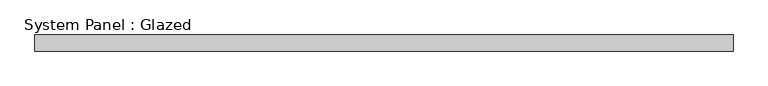
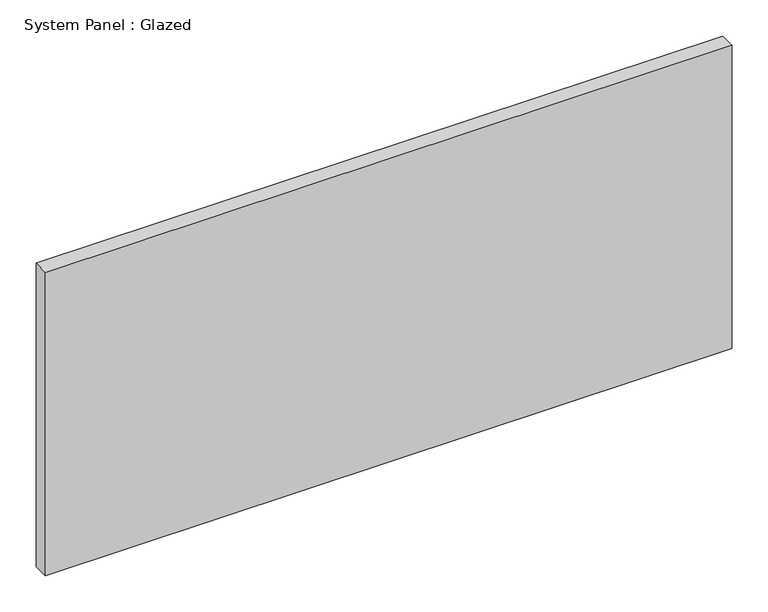
"""IFC4 building model written with IfcOpenShell, lengths in millimetres: plate geometry, System Panel : Glazed."""

from ifc_helpers import new_model, si_unit, origin, origin_with_axes, place, context, project, spatial, polyline, outline, extrude, source, transform, mapped, element, save


def system_panel_glazed_4b7b4477(model_context):
    return source(origin(), model_context, "Body", "SweptSolid", [
        extrude(outline(polyline([(550.3333332, 19.05), (-550.3333332, 19.05), (-550.3333332, 44.45), (550.3333332, 44.45), (550.3333332, 19.05)])), origin_with_axes(), (0.0, 0.0, 1.0), 514.35),
    ])


if __name__ == "__main__":
    model = new_model("IFC4")
    model_context = context("Model", 3, world=origin())
    ifc_project = project(units=[si_unit("LENGTHUNIT", "METRE", prefix="MILLI")], contexts=[model_context])
    site = spatial("IfcSite", under=ifc_project)
    building = spatial("IfcBuilding", under=site)
    placement = place(None, origin())
    system_panel_glazed_shape = system_panel_glazed_4b7b4477(model_context)
    element("IfcPlate", 1, ObjectType="System Panel : Glazed", at=placement, inside=building, context=model_context, shape_type="MappedRepresentation", body=[
        mapped(system_panel_glazed_shape, transform((0.0, 0.0, 0.0), x_axis=(1.0, 0.0, 0.0), y_axis=(0.0, 1.0, 0.0), z_axis=(0.0, 0.0, 1.0))),
    ])
    save(model, "model.ifc")

# Revit data of these elements
# Type "System Panel : Glazed"
#   Construction Type Id = "GSP4R"
#   Analytic Construction = "1/8 in Pilkington single glazing"
#   Visual Light Transmittance = 0.9
#   Solar Heat Gain Coefficient = 0.86
#   Heat Transfer Coefficient (U) = 1.18115 BTU/(h·ft²·°F)
#   Define Thermal Properties by = 1
# Element 1 (IfcPlate, "System Panel : Glazed")
#   Materials on its faces: "Glass"
# Materials
#   "Glass": class "Glass", colour RGB 0 128 192, transparency 0.75, Description = "Soda Lime Glass", Cost = 0
